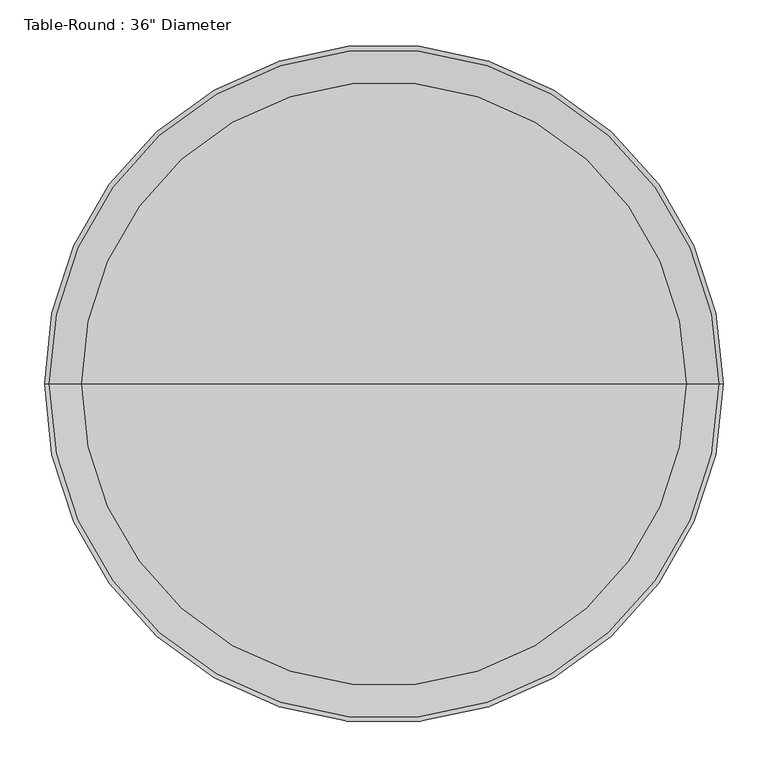
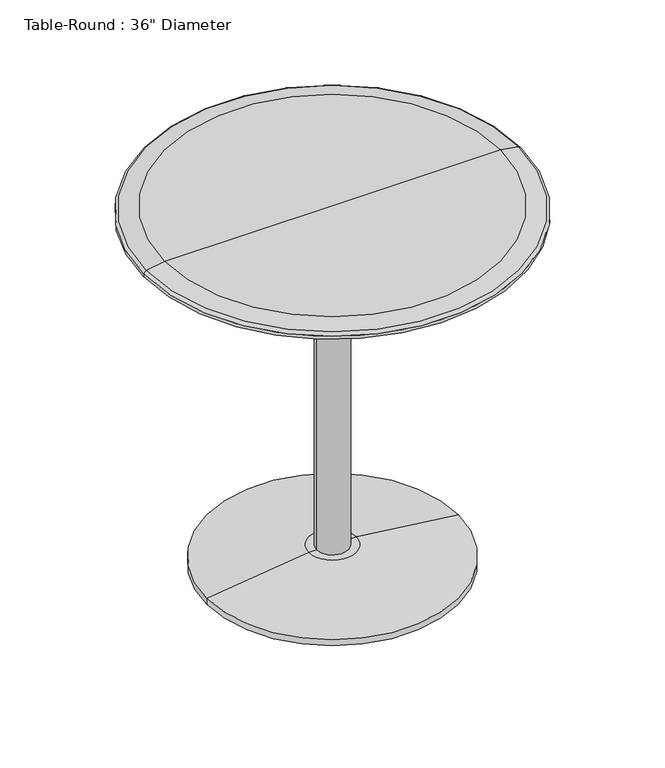
"""IFC4 building model written with IfcOpenShell, lengths in millimetres: furniture geometry."""

from ifc_helpers import new_model, si_unit, point, frame, origin, origin_2d, place, context, project, spatial, polyline, circle_curve, ellipse_curve, trimmed, segment, composite_curve, outline, extrude, source, transform, mapped, element, save
from ifc_brep_helpers import plane_surface, cylinder_surface, revolved_surface, advanced_brep


def furniture_ebfaaaa6(model_context):
    return source(origin(), model_context, "Body", "SolidModel", [
        extrude(outline(composite_curve([segment(trimmed(circle_curve(origin_2d(), 31.75), [point((-31.75, 0.0))], [point((31.75, 0.0))], False, "CARTESIAN"), True, "CONTINUOUS"), segment(trimmed(circle_curve(origin_2d(), 31.75), [point((31.75, 0.0))], [point((-31.75, 0.0))], False, "CARTESIAN"), True, "CONTINUOUS")], self_intersect=False)), frame((0.0, 0.0, 38.1), z_axis=(0.0, 0.0, 1.0), x_axis=(1.0, 0.0, 0.0)), (0.0, 0.0, 1.0), 704.85),
        advanced_brep(
        [(0.0, 0.0, 742.95), (-381.0, 0.0, 742.95), (381.0, 0.0, 742.95), (339.1011364, 0.0, 762.0), (-339.1011364, 0.0, 762.0), (0.0, 0.0, 762.0), (375.7526659, 0.0, 755.5373465), (-375.7526659, 0.0, 755.5373465), (381.0, 0.0, 749.2838172), (-381.0, 0.0, 749.2838172)],
        [
            (0, 1),
            (1, 2, circle_curve(frame((0.0, 0.0, 742.95), z_axis=(0.0, 0.0, -1.0), x_axis=(-1.0, 0.0, 0.0)), 381.0)),
            (2, 0),
            (2, 1, circle_curve(frame((0.0, 0.0, 742.95), z_axis=(0.0, 0.0, -1.0), x_axis=(-1.0, 0.0, 0.0)), 381.0)),
            (3, 4, circle_curve(frame((0.0, 0.0, 762.0), z_axis=(0.0, 0.0, 1.0), x_axis=(-1.0, 0.0, 0.0)), 339.1011364)),
            (4, 5),
            (5, 3),
            (4, 3, circle_curve(frame((0.0, 0.0, 762.0), z_axis=(0.0, 0.0, 1.0), x_axis=(-1.0, 0.0, 0.0)), 339.1011364)),
            (6, 7, circle_curve(frame((0.0, 0.0, 755.5373465), z_axis=(0.0, 0.0, 1.0), x_axis=(-1.0, 0.0, 0.0)), 375.7526659)),
            (7, 4),
            (3, 6),
            (7, 6, circle_curve(frame((0.0, 0.0, 755.5373465), z_axis=(0.0, 0.0, 1.0), x_axis=(-1.0, 0.0, 0.0)), 375.7526659)),
            (8, 9, circle_curve(frame((0.0, 0.0, 749.2838172), z_axis=(0.0, 0.0, 1.0), x_axis=(-1.0, 0.0, 0.0)), 381.0)),
            (9, 7, circle_curve(frame((-374.65, 0.0, 749.2838172), z_axis=(0.0, 1.0, 0.0), x_axis=(1.0, 0.0, 0.0)), 6.35)),
            (6, 8, circle_curve(frame((374.65, 0.0, 749.2838172), z_axis=(0.0, 1.0, 0.0), x_axis=(-1.0, 0.0, 0.0)), 6.35)),
            (9, 8, circle_curve(frame((0.0, 0.0, 749.2838172), z_axis=(0.0, 0.0, 1.0), x_axis=(-1.0, 0.0, 0.0)), 381.0)),
            (1, 9),
            (8, 2),
        ],
        [
            plane_surface(frame((0.0, 0.0, 742.95), z_axis=(0.0, 0.0, -1.0), x_axis=(-1.0, 0.0, 0.0))),
            plane_surface(frame((0.0, 0.0, 762.0), z_axis=(0.0, 0.0, 1.0), x_axis=(-1.0, 0.0, 0.0))),
            revolved_surface(polyline([(-339.1011364, 0.0, 762.0), (-375.7526659, 0.0, 755.5373465)]), (0.0, 0.0, 838.2), (0.0, 0.0, -1.0)),
            revolved_surface(trimmed(ellipse_curve(frame((-374.65, 0.0, 749.2838172), z_axis=(0.0, -1.0, 0.0), x_axis=(1.0, 0.0, 0.0)), 6.35, 6.35), [point((-375.7526659, 0.0, 755.5373465))], [point((-381.0, 0.0, 749.2838172))], True, "CARTESIAN"), (0.0, 0.0, 838.2), (0.0, 0.0, -1.0)),
            cylinder_surface(frame((0.0, 0.0, 838.2), z_axis=(0.0, 0.0, -1.0), x_axis=(-1.0, 0.0, 0.0)), 381.0),
        ],
        [
            (0, [[1, 2, 3]]),
            (0, [[-3, 4, -1]]),
            (1, [[5, 6, 7]]),
            (1, [[8, -7, -6]]),
            (2, [[9, 10, -5, 11]]),
            (2, [[12, -11, -8, -10]]),
            (3, [[13, 14, -9, 15]]),
            (3, [[16, -15, -12, -14]]),
            (4, [[-2, 17, -13, 18]]),
            (4, [[-4, -18, -16, -17]]),
        ],
    ),
        advanced_brep(
        [(0.0, 0.0, 0.0), (-254.0, 0.0, 0.0), (254.0, 0.0, 0.0), (47.625, 0.0, 38.1), (-47.625, 0.0, 38.1), (0.0, 0.0, 38.1), (254.0, 0.0, 12.7), (-254.0, 0.0, 12.7)],
        [
            (0, 1),
            (1, 2, circle_curve(frame((0.0, 0.0, 0.0), z_axis=(0.0, 0.0, -1.0), x_axis=(-1.0, 0.0, 0.0)), 254.0)),
            (2, 0),
            (2, 1, circle_curve(frame((0.0, 0.0, 0.0), z_axis=(0.0, 0.0, -1.0), x_axis=(-1.0, 0.0, 0.0)), 254.0)),
            (3, 4, circle_curve(frame((0.0, 0.0, 38.1), z_axis=(0.0, 0.0, 1.0), x_axis=(-1.0, 0.0, 0.0)), 47.625)),
            (4, 5),
            (5, 3),
            (4, 3, circle_curve(frame((0.0, 0.0, 38.1), z_axis=(0.0, 0.0, 1.0), x_axis=(-1.0, 0.0, 0.0)), 47.625)),
            (6, 7, circle_curve(frame((0.0, 0.0, 12.7), z_axis=(0.0, 0.0, 1.0), x_axis=(-1.0, 0.0, 0.0)), 254.0)),
            (7, 4),
            (3, 6),
            (7, 6, circle_curve(frame((0.0, 0.0, 12.7), z_axis=(0.0, 0.0, 1.0), x_axis=(-1.0, 0.0, 0.0)), 254.0)),
            (1, 7),
            (6, 2),
        ],
        [
            plane_surface(frame((0.0, 0.0, 0.0), z_axis=(0.0, 0.0, -1.0), x_axis=(-1.0, 0.0, 0.0))),
            plane_surface(frame((0.0, 0.0, 38.1), z_axis=(0.0, 0.0, 1.0), x_axis=(-1.0, 0.0, 0.0))),
            revolved_surface(polyline([(-47.625, 0.0, 38.1), (-254.0, 0.0, 12.7)]), (0.0, 0.0, 215.9), (0.0, 0.0, -1.0)),
            cylinder_surface(frame((0.0, 0.0, 215.9), z_axis=(0.0, 0.0, -1.0), x_axis=(-1.0, 0.0, 0.0)), 254.0),
        ],
        [
            (0, [[1, 2, 3]]),
            (0, [[-3, 4, -1]]),
            (1, [[5, 6, 7]]),
            (1, [[8, -7, -6]]),
            (2, [[9, 10, -5, 11]]),
            (2, [[12, -11, -8, -10]]),
            (3, [[-2, 13, -9, 14]]),
            (3, [[-4, -14, -12, -13]]),
        ],
    ),
    ])


if __name__ == "__main__":
    model = new_model("IFC4")
    model_context = context("Model", 3, world=origin())
    ifc_project = project(units=[si_unit("LENGTHUNIT", "METRE", prefix="MILLI")], contexts=[model_context])
    site = spatial("IfcSite", under=ifc_project)
    building = spatial("IfcBuilding", under=site)
    placement = place(None, origin())
    furniture_shape = furniture_ebfaaaa6(model_context)
    element("IfcFurniture", 1, ObjectType="Table-Round : 36\" Diameter", at=placement, inside=building, context=model_context, shape_type="MappedRepresentation", body=[
        mapped(furniture_shape, transform((0.0, 0.0, 0.0), x_axis=(1.0, 0.0, 0.0), y_axis=(0.0, 1.0, 0.0), z_axis=(0.0, 0.0, 1.0))),
    ])
    save(model, "model.ifc")

# Revit data of these elements
# Type "Table-Round : 36\" Diameter"
#   Assembly Code = "E2020200"
#   Base Radius = 0' - 10"
#   Height = 2' - 6"
#   Radius = 1' - 3"
#   Base Material = Steel, Chrome Plated
#   Top Material = Birch
#   Default Elevation = 0
# Element 1 (IfcFurniture, "Table-Round : 36\" Diameter")
#   Materials on its faces: "Steel, Chrome Plated", "Birch"
# Materials
#   "Steel, Chrome Plated": class "Metal", colour RGB 17 17 17, transparency 0, Description = "Chromiuim plated steel", Cost = 0
#   "Birch": class "Wood", colour RGB 224 178 126, transparency 0, Description = "Betula Alleghaniensis", Cost = 0
